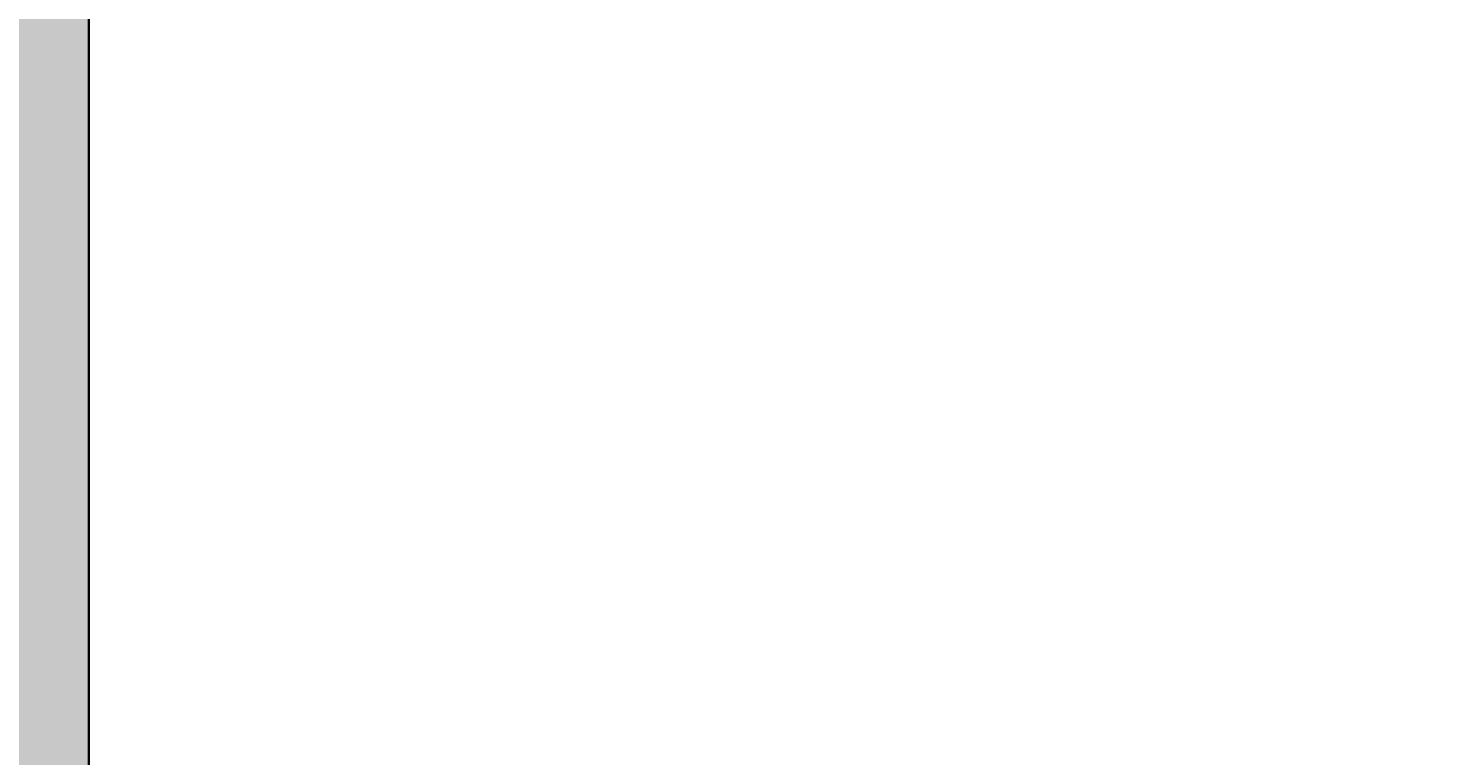
# Model space of a CAD drawing. Units: inches. Extents: x 1998 to 2588, y 1139 to 1977.
# Tile 77 of 134: x 2344 to 2397, y 1427 to 1454. Entities that reach past the tile are written whole.
import ezdxf

# ---------------------------------------------------------------- set-up
doc = ezdxf.new("R2010")
doc.units = ezdxf.units.IN
for name, color, linetype, lineweight in [('A-ANNO-DIMS', 2, 'Continuous', 18), ('A-WALL-PATT', 252, 'Continuous', 13), ('WALL', 200, 'Continuous', 35)]:
    doc.layers.add(name, color=color, linetype=linetype, lineweight=lineweight)
doc.styles.get("Standard").update_dxf_attribs({"font": 'arial.ttf'})
doc.dimstyles.get("Standard").update_dxf_attribs({"dimtxt": 0.18, "dimasz": 0.18, "dimexe": 0.18, "dimexo": 0.0625, "dimgap": 0.09, "dimtad": 0, "dimtih": 1, "dimtoh": 1, "dimdec": 4, "dimzin": 0, "dimdsep": 46, "dimtxsty": 'Standard', "dimcen": 0.09, "dimadec": 0, "dimazin": 0, "dimtfac": 1, "dimtdec": 4, "dimtofl": 0, "dimtmove": 0, "dimatfit": 3, "dimfxl": 1, "dimtolj": 1, "dimtzin": 0, "dimarcsym": 0})

# ---------------------------------------------------------------- blocks, each defined once
blk = doc.blocks.new('*D23')
at = {"layer": 'A-ANNO-DIMS', "color": 0, "lineweight": -2, "transparency": 16777216}
for p, q in [((2549.179, 1476.17), (2549.179, 1138.602)), ((2059.473, 1413.17), (2059.473, 1138.602)), ((2059.653, 1138.782), (2303.928, 1138.782)), ((2548.999, 1138.782), (2304.723, 1138.782))]:
    blk.add_line(p, q, dxfattribs=at)
at = {"layer": 'A-ANNO-DIMS', "color": 0, "transparency": 16777216}
for points in [[(2059.653, 1138.812), (2059.653, 1138.752), (2059.473, 1138.782)], [(2548.999, 1138.812), (2548.999, 1138.752), (2549.179, 1138.782)]]:
    blk.add_solid(points, dxfattribs=at)
at = {"layer": 'Defpoints', "color": 0, "transparency": 16777216}
for p in [(2549.179, 1476.232), (2059.473, 1413.232), (2549.179, 1138.782)]:
    blk.add_point(p, dxfattribs=at)
at = {"layer": 'A-ANNO-DIMS', "color": 0, "transparency": 16777216, "insert": (2304.326, 1138.782), "char_height": 0.18, "attachment_point": 5}
blk.add_mtext('\\A1;489.7', dxfattribs=at)
blk = doc.blocks.new('*D43')
at = {"layer": 'A-ANNO-DIMS', "color": 0, "lineweight": -2, "transparency": 16777216}
for p, q in [((2407.973, 1594.67), (2407.973, 1138.602)), ((2345.973, 1588.67), (2345.973, 1138.602)), ((2346.153, 1138.782), (2376.754, 1138.782)), ((2407.793, 1138.782), (2377.191, 1138.782))]:
    blk.add_line(p, q, dxfattribs=at)
at = {"layer": 'A-ANNO-DIMS', "color": 0, "transparency": 16777216}
for points in [[(2346.153, 1138.812), (2346.153, 1138.752), (2345.973, 1138.782)], [(2407.793, 1138.812), (2407.793, 1138.752), (2407.973, 1138.782)]]:
    blk.add_solid(points, dxfattribs=at)
at = {"layer": 'Defpoints', "color": 0, "transparency": 16777216}
for p in [(2407.973, 1594.732), (2345.973, 1588.732), (2407.973, 1138.782)]:
    blk.add_point(p, dxfattribs=at)
at = {"layer": 'A-ANNO-DIMS', "color": 0, "transparency": 16777216, "insert": (2376.973, 1138.782), "char_height": 0.18, "attachment_point": 5}
blk.add_mtext('\\A1;62', dxfattribs=at)

msp = doc.modelspace()

# ---------------------------------------------------------------- hatches: boundary and pattern name
at = {"layer": 'A-WALL-PATT'}
h = msp.add_hatch(color=256, dxfattribs=at)
h.dxf.hatch_style = 1
h.paths.add_polyline_path([(2222.9729, 1888.7324), (2099.4125, 1888.7324), (2099.4125, 1879.7324), (2222.9729, 1879.7324)])
h.paths.add_polyline_path([(2096.9729, 1868.3278), (2087.9729, 1868.3278), (2087.9729, 1775.637), (2096.9729, 1775.637)])
h.paths.add_polyline_path([(2227.4729, 1868.3278), (2222.9729, 1868.3278), (2222.9729, 1774.3318), (2227.4729, 1774.3318)])
h.paths.add_polyline_path([(2188.3019, 1759.7324), (2138.6074, 1759.7324), (2099.4125, 1759.7324), (2099.4125, 1755.2324), (2176.9729, 1755.2324), (2188.3019, 1755.2324)])
h.paths.add_polyline_path([(2087.9729, 1759.7324), (2059.4729, 1759.7324), (2059.4729, 1702.7324), (2087.9729, 1702.7324), (2087.9729, 1707.2324), (2063.9729, 1707.2324), (2063.9729, 1755.2324), (2087.9729, 1755.2324)])
h.paths.add_polyline_path([(2096.9729, 1755.2324), (2087.9729, 1755.2324), (2087.9729, 1707.2324), (2096.9729, 1707.2324)])
h.paths.add_polyline_path([(2187.0461, 1707.2324), (2105.9729, 1707.2324), (2096.9729, 1707.2324), (2087.9729, 1707.2324), (2087.9729, 1702.7324), (2105.9729, 1702.7324), (2114.9729, 1702.7324), (2187.0461, 1702.7324)])
h.paths.add_polyline_path([(2181.4729, 1719.2028), (2176.9729, 1719.2028), (2176.9729, 1707.2324), (2181.4729, 1707.2324)])
h.paths.add_polyline_path([(2216.0332, 1588.7324), (2114.9729, 1588.7324), (2105.9729, 1588.7324), (2105.9729, 1584.2324), (2216.0332, 1584.2324)])
h.paths.add_polyline_path([(2077.691, 1588.7324), (2061.4729, 1588.7324), (2061.4729, 1584.2324), (2077.691, 1584.2324)])
h.paths.add_polyline_path([(2105.9729, 1588.7324), (2098.0956, 1588.7324), (2098.0956, 1584.2324), (2105.9729, 1584.2324)])
h.paths.add_polyline_path([(2114.9729, 1596.2642), (2110.1012, 1596.2642), (2105.9729, 1596.2642), (2105.9729, 1588.7324), (2114.9729, 1588.7324)])
h.paths.add_polyline_path([(2114.9729, 1584.2324), (2105.9729, 1584.2324), (2105.9729, 1580.249), (2110.1012, 1580.249), (2114.9729, 1580.249)])
h.paths.add_polyline_path([(2114.9729, 1547.7716), (2110.1012, 1547.7716, -0.0318759), (2105.9729, 1548.035), (2105.9729, 1470.2324), (2108.3775, 1470.2324), (2108.3775, 1465.7324), (2186.2943, 1465.7324), (2186.2943, 1470.2324), (2114.9729, 1470.2324)])
h.paths.add_polyline_path([(2227.4729, 1584.2324), (2222.9729, 1584.2324), (2222.9729, 1486.137), (2227.4729, 1486.137)])
h.paths.add_polyline_path([(2295.4138, 1593.2324), (2227.4729, 1593.2324), (2227.4729, 1588.7324), (2295.4138, 1588.7324), (2295.4138, 1591.8729)])
h.paths.add_polyline_path([(2345.9729, 1627.1165), (2341.4729, 1627.1165), (2341.4729, 1593.2324), (2337.2869, 1593.2324), (2337.2869, 1591.8729), (2337.2869, 1588.7324), (2345.9729, 1588.7324)])
h.paths.add_polyline_path([(2291.9729, 1588.7324), (2287.4729, 1588.7324), (2287.4729, 1522.7324), (2291.9729, 1522.7324)])
h.paths.add_polyline_path([(2291.9729, 1522.7324), (2287.4729, 1522.7324), (2227.4729, 1522.7324), (2227.4729, 1518.2324), (2291.9729, 1518.2324)])
h.paths.add_polyline_path([(2295.7347, 1519.5919), (2295.7347, 1522.7324), (2291.9729, 1522.7324), (2291.9729, 1518.2324), (2295.7347, 1518.2324)])
h.paths.add_polyline_path([(2345.9729, 1522.7324), (2337.6078, 1522.7324), (2337.6078, 1519.5919), (2337.6078, 1518.2324), (2341.4729, 1518.2324), (2341.4729, 1488.5616), (2345.9729, 1488.5616)])
h.paths.add_polyline_path([(2345.9729, 1468.1569), (2341.4729, 1468.1569), (2341.4729, 1374.2324), (2227.4729, 1374.2324), (2227.4729, 1369.7324), (2345.9729, 1369.7324)])
h.paths.add_polyline_path([(2345.9729, 1369.7324), (2341.4729, 1369.7324), (2341.4729, 1362.2324), (2345.9729, 1362.2324)])
h.paths.add_polyline_path([(2345.9729, 1317.7324), (2345.9729, 1322.2324), (2341.4729, 1322.2324), (2341.4729, 1285.137), (2345.9729, 1285.137)], flags=17)
h.paths.add_polyline_path([(2356.2096, 1322.2324), (2345.9729, 1322.2324), (2345.9729, 1317.7324), (2356.2096, 1317.7324), (2356.2096, 1319.3088)], flags=17)
h.paths.add_polyline_path([(2393.9729, 1322.2324), (2375.6999, 1322.2324), (2375.6999, 1319.3088, -0.0202458), (2375.636, 1317.7324), (2393.9729, 1317.7324)], flags=17)
h.paths.add_polyline_path([(2398.4729, 1322.2324), (2393.9729, 1322.2324), (2393.9729, 1317.7324), (2393.9729, 1237.7324), (2345.9729, 1237.7324), (2345.9729, 1264.7324), (2341.4729, 1264.7324), (2341.4729, 1228.7324), (2393.9729, 1228.7324), (2482.7412, 1228.7324), (2482.7412, 1237.7324), (2398.4729, 1237.7324), (2398.4729, 1297.1029)])
h.paths.add_polyline_path([(2398.4729, 1362.2324), (2393.9729, 1362.2324), (2393.9729, 1357.7324), (2398.4729, 1357.7324)])
h.paths.add_polyline_path([(2345.9729, 1329.7549), (2341.4729, 1329.7549), (2341.4729, 1322.2324), (2345.9729, 1322.2324)])

# ---------------------------------------------------------------- linework, layer by layer
at = {"layer": 'WALL'}
msp.add_line((2345.9729, 1522.7324), (2345.9729, 1369.7324), dxfattribs=at)

# ---------------------------------------------------------------- dimensions: what is measured, and where the dimension line sits
at = {"layer": 'A-ANNO-DIMS'}
for base, p1, p2, override, picture, middle in [((2407.9729, 1138.7824), (2345.9729, 1588.7324), (2407.9729, 1594.7324), {"dimdec": 0, "dimlfac": 1, "dimrnd": 0, "dimzin": 0, "dimdsep": 46, "dimlunit": 2}, '*D43', (2376.9729, 1138.7824)), ((2549.1786, 1138.7824), (2059.4729, 1413.2324), (2549.1786, 1476.2324), {"dimdec": 1, "dimlfac": 1, "dimrnd": 0, "dimzin": 0, "dimdsep": 46, "dimlunit": 2}, '*D23', (2304.3257, 1138.7824))]:
    dim = msp.add_linear_dim(base=base, p1=p1, p2=p2, dimstyle='Standard', override=override, dxfattribs=at)
    dim.commit()
    dim.dimension.update_dxf_attribs({"geometry": picture, "text_midpoint": middle})

doc.saveas('drawing.dxf')
